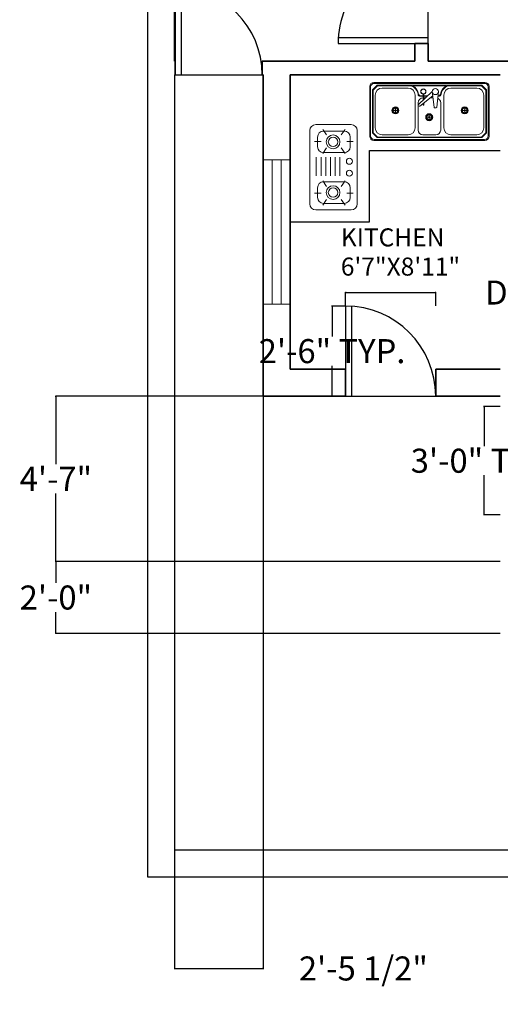
# Model space of a CAD drawing. Units: inches. Extents: x -11 to 443, y 65 to 743.
# Tile 1 of 10: x 2 to 162, y 65 to 392. Entities that reach past the tile are written whole.
import ezdxf

# ---------------------------------------------------------------- set-up
doc = ezdxf.new("R2010")
doc.units = ezdxf.units.IN
doc.header["$MEASUREMENT"] = 0
for name, color, linetype, lineweight in [('A-ANNO-DIMS', 2, 'Continuous', 18), ('A-AREA-IDEN', 2, 'Continuous', 18), ('A-DOOR', 4, 'Continuous', 25), ('A-EQPM', 8, 'Continuous', 18), ('A-FLOR-CASE', 8, 'Continuous', 25), ('A-FLOR-FIXT', 8, 'Continuous', 18), ('A-GLAZ', 4, 'Continuous', 18), ('A-WALL', 7, 'Continuous', 35), ('A-WALL-SITE', 7, 'Continuous', 30), ('C-PROP', 3, 'Continuous', 30)]:
    doc.layers.add(name, color=color, linetype=linetype, lineweight=lineweight)
doc.styles.get("Standard").update_dxf_attribs({"font": 'italic8.shx'})
doc.dimstyles.get("Standard").update_dxf_attribs({"dimtxt": 8, "dimasz": 0.18, "dimexe": 0.18, "dimexo": 0.0625, "dimgap": 0.09, "dimtad": 0, "dimtih": 1, "dimtoh": 1, "dimzin": 0, "dimdsep": 46, "dimlunit": 3, "dimtxsty": 'Standard', "dimblk": 'CLOSEDBLANK', "dimcen": 0.09, "dimclrd": 6, "dimclre": 5, "dimclrt": 4, "dimadec": 0, "dimazin": 0, "dimtfac": 1, "dimtofl": 0, "dimtmove": 0, "dimatfit": 3, "dimfxl": 1, "dimtolj": 1, "dimtzin": 0, "dimarcsym": 0})

# ---------------------------------------------------------------- blocks, each defined once
blk = doc.blocks.new('DOOR-SWING-30')
for p, q in [((0, 30), (0, 0)), ((2, 29.93), (2, 0)), ((0, 0), (30, 0))]:
    blk.add_line(p, q)
blk.add_arc((0, 0), 30, 0, 90)
blk = doc.blocks.new('WIN-48x9')
for p, q in [((0, 48), (0, 0)), ((9, 48), (0, 48)), ((3, 0), (3, 48)), ((6, 0), (6, 48)), ((9, 0), (9, 48)), ((0, 0), (9, 0))]:
    blk.add_line(p, q)
blk = doc.blocks.new('_ClosedBlank')
at = {"color": 0, "linetype": 'ByBlock', "lineweight": -2}
for p, q in [((-1, 0.17), (0, 0)), ((-1, 0.17), (-1, -0.17)), ((0, 0), (-1, -0.17))]:
    blk.add_line(p, q, dxfattribs=at)
blk = doc.blocks.new('*D20')
at = {"layer": 'A-ANNO-DIMS', "color": 5, "lineweight": -2, "transparency": 16777216}
for p, q in [((110.2, 296.98), (110.2, 301.6)), ((140.2, 296.98), (140.2, 301.6))]:
    blk.add_line(p, q, dxfattribs=at)
at = {"layer": 'A-ANNO-DIMS', "color": 6, "lineweight": -2, "transparency": 16777216}
for p, q in [((110.38, 301.42), (140.02, 301.42)), ((140.2, 301.42), (140.38, 301.42))]:
    blk.add_line(p, q, dxfattribs=at)
at = {"layer": 'Defpoints', "color": 0, "lineweight": 100, "transparency": 16777216}
for p in [(140.2, 301.42), (110.2, 296.92), (140.2, 296.92)]:
    blk.add_point(p, dxfattribs=at)
at = {"layer": 'A-ANNO-DIMS', "color": 6, "lineweight": -2, "transparency": 16777216, "xscale": 0.18, "yscale": 0.18, "zscale": 0.18, "rotation": 180}
blk.add_blockref('_ClosedBlank', (110.2, 301.42), dxfattribs=at)
at = {"layer": 'A-ANNO-DIMS', "color": 6, "lineweight": -2, "transparency": 16777216, "xscale": 0.18, "yscale": 0.18, "zscale": 0.18}
blk.add_blockref('_ClosedBlank', (140.2, 301.42), dxfattribs=at)
at = {"layer": 'A-ANNO-DIMS', "color": 4, "transparency": 16777216, "insert": (197.61, 301.42), "char_height": 8, "attachment_point": 5}
blk.add_mtext('\\A1;DOOR 2\'-6" TYP.', dxfattribs=at)
blk = doc.blocks.new('*D21')
at = {"layer": 'A-ANNO-DIMS', "color": 5, "lineweight": -2, "transparency": 16777216}
for p, q in [((110.14, 296.92), (105.52, 296.92)), ((110.14, 266.92), (105.52, 266.92))]:
    blk.add_line(p, q, dxfattribs=at)
at = {"layer": 'A-ANNO-DIMS', "color": 6, "lineweight": -2, "transparency": 16777216}
for p, q in [((105.7, 296.74), (105.7, 286.77)), ((105.7, 267.1), (105.7, 277.07))]:
    blk.add_line(p, q, dxfattribs=at)
at = {"layer": 'Defpoints', "color": 0, "lineweight": 100, "transparency": 16777216}
for p in [(105.7, 296.92), (110.2, 296.92), (110.2, 266.92)]:
    blk.add_point(p, dxfattribs=at)
at = {"layer": 'A-ANNO-DIMS', "color": 6, "lineweight": -2, "transparency": 16777216, "xscale": 0.18, "yscale": 0.18, "zscale": 0.18}
for p, rotation in [((105.7, 296.92), 90), ((105.7, 266.92), 270)]:
    blk.add_blockref('_ClosedBlank', p, dxfattribs=dict(at, rotation=rotation))
at = {"layer": 'A-ANNO-DIMS', "color": 4, "transparency": 16777216, "insert": (105.7, 281.92), "char_height": 8, "attachment_point": 5}
blk.add_mtext('\\A1;2\'-6" TYP.', dxfattribs=at)
blk = doc.blocks.new('*D23')
at = {"layer": 'A-ANNO-DIMS', "color": 5, "lineweight": -2, "transparency": 16777216}
for p, q in [((161.65, 263.44), (156.13, 263.44)), ((161.65, 227.44), (156.13, 227.44))]:
    blk.add_line(p, q, dxfattribs=at)
at = {"layer": 'A-ANNO-DIMS', "color": 6, "lineweight": -2, "transparency": 16777216}
for p, q in [((156.31, 263.26), (156.31, 250.29)), ((156.31, 227.62), (156.31, 240.59))]:
    blk.add_line(p, q, dxfattribs=at)
at = {"layer": 'Defpoints', "color": 0, "lineweight": 100, "transparency": 16777216}
for p in [(156.31, 263.44), (161.71, 263.44), (161.71, 227.44)]:
    blk.add_point(p, dxfattribs=at)
at = {"layer": 'A-ANNO-DIMS', "color": 6, "lineweight": -2, "transparency": 16777216, "xscale": 0.18, "yscale": 0.18, "zscale": 0.18}
for p, rotation in [((156.31, 263.44), 90), ((156.31, 227.44), 270)]:
    blk.add_blockref('_ClosedBlank', p, dxfattribs=dict(at, rotation=rotation))
at = {"layer": 'A-ANNO-DIMS', "color": 4, "transparency": 16777216, "insert": (156.31, 245.44), "char_height": 8, "attachment_point": 5}
blk.add_mtext('\\A1;3\'-0" TYP.', dxfattribs=at)
blk = doc.blocks.new('*D37')
at = {"layer": 'A-ANNO-DIMS', "color": 5, "lineweight": -2, "transparency": 16777216}
for p, q in [((53.21, 373.86), (53.21, 76.28)), ((82.71, 266.86), (82.71, 76.28))]:
    blk.add_line(p, q, dxfattribs=at)
at = {"layer": 'A-ANNO-DIMS', "color": 6, "lineweight": -2, "transparency": 16777216}
for p, q in [((53.39, 76.46), (82.53, 76.46)), ((82.71, 76.46), (82.89, 76.46))]:
    blk.add_line(p, q, dxfattribs=at)
at = {"layer": 'Defpoints', "color": 0, "lineweight": 100, "transparency": 16777216}
for p in [(53.21, 373.92), (82.71, 266.92), (82.71, 76.46)]:
    blk.add_point(p, dxfattribs=at)
at = {"layer": 'A-ANNO-DIMS', "color": 6, "lineweight": -2, "transparency": 16777216, "xscale": 0.18, "yscale": 0.18, "zscale": 0.18, "rotation": 180}
blk.add_blockref('_ClosedBlank', (53.21, 76.46), dxfattribs=at)
at = {"layer": 'A-ANNO-DIMS', "color": 6, "lineweight": -2, "transparency": 16777216, "xscale": 0.18, "yscale": 0.18, "zscale": 0.18}
blk.add_blockref('_ClosedBlank', (82.71, 76.46), dxfattribs=at)
at = {"layer": 'A-ANNO-DIMS', "color": 4, "transparency": 16777216, "insert": (116.12, 76.46), "char_height": 8, "attachment_point": 5}
blk.add_mtext('\\A1;2\'-5 1/2"', dxfattribs=at)
blk = doc.blocks.new('*D38')
at = {"layer": 'A-ANNO-DIMS', "color": 5, "lineweight": -2, "transparency": 16777216}
for p, q in [((82.65, 266.92), (13.57, 266.92)), ((161.65, 211.92), (13.57, 211.92))]:
    blk.add_line(p, q, dxfattribs=at)
at = {"layer": 'A-ANNO-DIMS', "color": 6, "lineweight": -2, "transparency": 16777216}
for p, q in [((13.75, 266.74), (13.75, 244.27)), ((13.75, 212.1), (13.75, 234.57))]:
    blk.add_line(p, q, dxfattribs=at)
at = {"layer": 'Defpoints', "color": 0, "lineweight": 100, "transparency": 16777216}
for p in [(82.71, 266.92), (13.75, 211.92), (161.71, 211.92)]:
    blk.add_point(p, dxfattribs=at)
at = {"layer": 'A-ANNO-DIMS', "color": 6, "lineweight": -2, "transparency": 16777216, "xscale": 0.18, "yscale": 0.18, "zscale": 0.18}
for p, rotation in [((13.75, 266.92), 90), ((13.75, 211.92), 270)]:
    blk.add_blockref('_ClosedBlank', p, dxfattribs=dict(at, rotation=rotation))
at = {"layer": 'A-ANNO-DIMS', "color": 4, "transparency": 16777216, "insert": (13.75, 239.42), "char_height": 8, "attachment_point": 5}
blk.add_mtext('\\A1;4\'-7"', dxfattribs=at)
blk = doc.blocks.new('*D39')
at = {"layer": 'A-ANNO-DIMS', "color": 5, "lineweight": -2, "transparency": 16777216}
for p, q in [((161.65, 211.92), (13.57, 211.92)), ((161.65, 187.92), (13.57, 187.92))]:
    blk.add_line(p, q, dxfattribs=at)
at = {"layer": 'A-ANNO-DIMS', "color": 6, "lineweight": -2, "transparency": 16777216}
for p, q in [((13.75, 211.74), (13.75, 204.77)), ((13.75, 188.1), (13.75, 195.07))]:
    blk.add_line(p, q, dxfattribs=at)
at = {"layer": 'Defpoints', "color": 0, "lineweight": 100, "transparency": 16777216}
for p in [(161.71, 211.92), (13.75, 187.92), (161.71, 187.92)]:
    blk.add_point(p, dxfattribs=at)
at = {"layer": 'A-ANNO-DIMS', "color": 6, "lineweight": -2, "transparency": 16777216, "xscale": 0.18, "yscale": 0.18, "zscale": 0.18}
for p, rotation in [((13.75, 211.92), 90), ((13.75, 187.92), 270)]:
    blk.add_blockref('_ClosedBlank', p, dxfattribs=dict(at, rotation=rotation))
at = {"layer": 'A-ANNO-DIMS', "color": 4, "transparency": 16777216, "insert": (13.75, 199.92), "char_height": 8, "attachment_point": 5}
blk.add_mtext('\\A1;2\'-0"', dxfattribs=at)

msp = doc.modelspace()

# ---------------------------------------------------------------- linework, layer by layer
at = {"layer": 'A-DOOR'}
for p, q in [((53.43, 402.92), (53.43, 373.92)), ((55.43, 402.851), (55.43, 373.92)), ((53.43, 373.92), (82.43, 373.92))]:
    msp.add_line(p, q, dxfattribs=at)
msp.add_arc((53.43, 373.92), 29, 0, 90, dxfattribs=at)
at = {"layer": 'A-EQPM'}
for p, q in [((100.263, 357.301), (112.074, 357.301)), ((98.294, 330.923), (98.294, 355.333)), ((102.588, 355.724), (103.876, 353.86)), ((102.838, 355.15), (109.783, 355.15)), ((110.033, 355.724), (108.744, 353.86)), ((114.042, 355.333), (114.042, 330.923)), ((99.867, 351.709), (102.015, 351.709)), ((100.869, 349.949), (100.869, 353.182)), ((112.754, 351.709), (110.606, 351.709)), ((111.751, 353.182), (111.751, 349.949)), ((102.588, 347.694), (103.876, 349.558)), ((109.783, 347.981), (102.838, 347.981)), ((110.033, 347.694), (108.744, 349.558)), ((100.44, 340.283), (100.44, 346.449)), ((102.015, 340.283), (102.015, 346.449)), ((103.589, 340.283), (103.589, 346.449)), ((105.164, 340.283), (105.164, 346.449)), ((106.739, 340.283), (106.739, 346.449)), ((108.314, 340.283), (108.314, 346.449)), ((102.588, 338.562), (103.876, 336.698)), ((109.783, 338.275), (102.838, 338.275)), ((110.033, 338.562), (108.744, 336.698)), ((99.867, 334.547), (102.015, 334.547)), ((100.869, 336.307), (100.869, 333.074)), ((112.754, 334.547), (110.606, 334.547)), ((111.751, 333.074), (111.751, 336.307)), ((102.588, 330.532), (103.876, 332.396)), ((102.838, 331.106), (109.783, 331.106)), ((110.033, 330.532), (108.744, 332.396)), ((112.074, 328.955), (100.263, 328.955))]:
    msp.add_line(p, q, dxfattribs=at)
for centre, radius in [((106.024, 351.566), 2.294), ((106.024, 351.566), 1.577), ((111.465, 345.113), 1.004), ((111.465, 341.143), 1.004), ((106.024, 334.691), 2.294), ((106.024, 334.691), 1.577)]:
    msp.add_circle(centre, radius, dxfattribs=at)
for centre, start, end in [((100.263, 355.333), 90, 180), ((112.074, 355.333), 0, 90), ((102.838, 353.182), 90, 180), ((109.783, 353.182), 0, 90), ((102.838, 349.949), 180, 270), ((109.783, 349.949), 270, 0), ((102.838, 336.307), 90, 180), ((109.783, 336.307), 0, 90), ((102.838, 333.074), 180, 270), ((109.783, 333.074), 270, 0), ((100.263, 330.923), 180, 270), ((112.074, 330.923), 270, 0)]:
    msp.add_arc(centre, 1.968, start, end, dxfattribs=at)
at = {"layer": 'A-FLOR-CASE'}
for p, q in [((118.155, 324.92), (118.155, 348.71)), ((118.155, 348.71), (161.709, 348.71)), ((91.709, 324.92), (91.709, 324.92)), ((91.709, 324.92), (118.155, 324.92))]:
    msp.add_line(p, q, dxfattribs=at)
at = {"layer": 'A-FLOR-FIXT'}
for p, q in [((120.702, 370.454), (119.127, 368.879)), ((156.607, 371.36), (119.599, 371.36)), ((156.489, 371.045), (119.718, 371.045)), ((155.505, 370.454), (120.702, 370.454)), ((157.08, 368.879), (155.505, 370.454)), ((118.221, 369.982), (118.221, 353.446)), ((118.536, 369.864), (118.536, 353.564)), ((119.127, 368.879), (119.127, 354.549)), ((120.783, 370.257), (119.324, 368.798)), ((119.324, 368.798), (119.324, 354.63)), ((120.054, 367.106), (120.054, 356.263)), ((132.049, 370.257), (120.783, 370.257)), ((130.992, 369.469), (122.416, 369.469)), ((143.821, 370.257), (132.51, 370.257)), ((133.354, 356.263), (133.354, 367.106)), ((139.065, 368.32), (134.493, 363.973)), ((135.98, 365.387), (135.98, 367.447)), ((136.226, 367.452), (136.226, 365.621)), ((139.065, 368.32), (139.64, 363.091)), ((140.598, 363.093), (141.117, 368.32)), ((142.9, 367.106), (142.9, 356.263)), ((155.423, 370.257), (144.283, 370.257)), ((153.838, 369.469), (145.263, 369.469)), ((156.883, 368.798), (155.423, 370.257)), ((156.201, 356.263), (156.201, 367.106)), ((156.883, 354.63), (156.883, 368.798)), ((157.08, 354.549), (157.08, 368.879)), ((157.67, 353.564), (157.67, 369.864)), ((157.985, 353.446), (157.985, 369.982)), ((134.356, 364.61), (134.356, 355.478)), ((139.227, 366.841), (134.924, 363.473)), ((135.98, 366.938), (135.095, 366.938)), ((135.98, 366.741), (135.095, 366.741)), ((135.98, 366.185), (135.931, 366.185)), ((135.98, 363.759), (135.98, 364.299)), ((136.226, 363.759), (135.98, 363.759)), ((137.612, 366.938), (136.226, 366.938)), ((137.405, 366.741), (136.226, 366.741)), ((136.819, 366.185), (136.226, 366.185)), ((136.226, 364.492), (136.226, 363.759)), ((139.3, 366.185), (138.389, 366.185)), ((139.238, 366.741), (139.1, 366.741)), ((141.237, 366.741), (140.96, 366.741)), ((141.237, 366.938), (140.98, 366.938)), ((141.862, 355.478), (141.862, 364.61)), ((126.58, 362.025), (125.989, 362.025)), ((126.784, 362.229), (126.784, 362.819)), ((126.784, 361.821), (126.784, 361.23)), ((126.988, 362.025), (127.578, 362.025)), ((134.486, 363.521), (134.466, 363.545)), ((138.031, 359.981), (138.031, 360.571)), ((139.836, 362.916), (140.402, 362.915)), ((149.638, 362.025), (149.047, 362.025)), ((149.842, 362.229), (149.842, 362.819)), ((149.842, 361.821), (149.842, 361.23)), ((150.045, 362.025), (150.636, 362.025)), ((137.828, 359.777), (137.237, 359.777)), ((138.031, 359.573), (138.031, 358.982)), ((138.235, 359.777), (138.826, 359.777)), ((119.127, 354.549), (120.702, 352.974)), ((119.324, 354.63), (120.783, 353.171)), ((155.423, 353.171), (156.883, 354.63)), ((155.505, 352.974), (157.08, 354.549)), ((119.599, 352.068), (156.607, 352.068)), ((119.718, 352.383), (156.489, 352.383)), ((120.702, 352.974), (155.505, 352.974)), ((120.783, 353.171), (155.423, 353.171)), ((122.416, 353.9), (130.992, 353.9)), ((135.931, 353.903), (140.288, 353.903)), ((145.263, 353.9), (153.838, 353.9))]:
    msp.add_line(p, q, dxfattribs=at)
for centre, radius in [((136.083, 368.307), 0.866), ((136.083, 368.307), 0.787), ((140.091, 368.32), 1.026), ((126.784, 362.025), 1.162), ((126.784, 362.025), 1.099), ((126.784, 362.025), 0.83), ((126.784, 362.025), 0.794), ((126.784, 362.025), 0.204), ((126.784, 362.025), 0.0958), ((138.031, 359.777), 1.162), ((138.031, 359.777), 1.099), ((138.031, 359.777), 0.83), ((138.031, 359.777), 0.794), ((149.842, 362.025), 1.162), ((149.842, 362.025), 1.099), ((149.842, 362.025), 0.83), ((149.842, 362.025), 0.794), ((149.842, 362.025), 0.204), ((149.842, 362.025), 0.0958), ((138.031, 359.777), 0.204), ((138.031, 359.777), 0.0958)]:
    msp.add_circle(centre, radius, dxfattribs=at)
for centre, radius, start, end in [((119.599, 369.982), 1.378, 90, 180), ((119.718, 369.864), 1.181, 90, 180), ((156.489, 369.864), 1.181, 0, 90), ((156.607, 369.982), 1.378, 0, 90), ((122.416, 367.106), 2.362, 90, 180), ((130.992, 367.106), 2.362, 0, 90), ((130.657, 366.822), 3.706, 9.04683, 67.9454), ((130.657, 366.822), 3.903, 9.04683, 61.65237), ((135.095, 367.529), 0.787, 189.04683, 270), ((135.095, 367.529), 0.591, 189.04683, 270), ((141.237, 367.529), 0.591, 270, 350.95317), ((141.237, 367.529), 0.787, 270, 350.95317), ((145.674, 366.822), 3.903, 118.34763, 170.95317), ((145.674, 366.822), 3.706, 112.0546, 170.95317), ((145.263, 367.106), 2.362, 90, 180), ((153.838, 367.106), 2.362, 0, 90), ((135.931, 364.61), 1.575, 90, 180), ((134.71, 363.745), 0.315, 133.56108, 219.26187), ((140.288, 364.61), 1.575, 360, 67.38374), ((134.73, 363.721), 0.315, 219.26187, 308.04948), ((139.836, 363.113), 0.197, 186.28076, 269.95427), ((140.402, 363.112), 0.197, 269.95427, 354.32947), ((122.416, 356.263), 2.362, 180, 270), ((130.992, 356.263), 2.362, 270, 0), ((135.931, 355.478), 1.575, 180, 270), ((140.288, 355.478), 1.575, 270, 0), ((145.263, 356.263), 2.362, 180, 270), ((153.838, 356.263), 2.362, 270, 0), ((119.599, 353.446), 1.378, 180, 270), ((119.718, 353.564), 1.181, 180, 270), ((156.489, 353.564), 1.181, 270, 360), ((156.607, 353.446), 1.378, 270, 360)]:
    msp.add_arc(centre, radius, start, end, dxfattribs=at)
at = {"layer": 'A-WALL'}
for p, q in [((53.209, 517.92), (53.209, 378.42)), ((137.709, 384.35), (133.209, 384.35)), ((133.209, 384.35), (133.209, 378.42)), ((137.709, 384.35), (137.709, 378.42)), ((53.209, 378.42), (53.43, 378.42)), ((53.43, 373.92), (53.43, 378.42)), ((82.43, 373.92), (82.43, 378.42)), ((82.43, 378.42), (133.209, 378.42)), ((137.709, 378.42), (169.908, 378.42)), ((53.209, 373.92), (53.43, 373.92)), ((82.709, 373.92), (82.43, 373.92)), ((82.43, 373.92), (82.709, 373.92)), ((82.709, 266.92), (82.709, 373.92)), ((91.709, 275.92), (91.709, 373.92)), ((91.709, 373.92), (161.709, 373.92)), ((91.709, 275.92), (110.201, 275.92)), ((110.201, 275.92), (110.201, 266.92)), ((140.201, 275.92), (140.201, 266.92)), ((140.201, 275.92), (161.709, 275.92)), ((82.709, 266.92), (110.201, 266.92)), ((140.201, 266.92), (161.709, 266.92))]:
    msp.add_line(p, q, dxfattribs=at)
at = {"layer": 'A-WALL-SITE'}
for p, q in [((53.209, 373.92), (53.209, 115.92)), ((53.209, 115.92), (323.209, 115.92))]:
    msp.add_line(p, q, dxfattribs=at)
at = {"layer": 'C-PROP'}
msp.add_lwpolyline([(44.209, 106.92), (332.209, 106.92), (332.209, 706.92), (44.209, 706.92)], close=True, dxfattribs=at)

# ---------------------------------------------------------------- block references
at = {"layer": 'A-DOOR', "rotation": 89.99999999999991}
msp.add_blockref('DOOR-SWING-30', (137.709, 384.35), dxfattribs=at)
at = {"layer": 'A-DOOR'}
msp.add_blockref('DOOR-SWING-30', (110.201, 266.92), dxfattribs=at)
at = {"layer": 'A-GLAZ'}
msp.add_blockref('WIN-48x9', (82.709, 297.576), dxfattribs=at)

# ---------------------------------------------------------------- texts
at = {"layer": 'A-AREA-IDEN'}
for s, p in [('KITCHEN', (108.605, 316.776)), ('6\'7"X8\'11"', (108.605, 307.062))]:
    msp.add_text(s, height=6, dxfattribs=at).set_placement(p)

# ---------------------------------------------------------------- dimensions: what is measured, and where the dimension line sits
at = {"layer": 'A-ANNO-DIMS'}
dim = msp.add_linear_dim(base=(82.709, 76.46), p1=(53.209, 373.92), p2=(82.709, 266.92), dimstyle='Standard', override={"dimdec": 1, "dimlfac": 1, "dimrnd": 0, "dimzin": 1, "dimdsep": 46, "dimlunit": 4, "dimfrac": 2}, dxfattribs=at)
dim.commit()
dim.dimension.update_dxf_attribs({"geometry": '*D37', "text_midpoint": (116.122, 76.46)})
dim = msp.add_linear_dim(base=(140.201, 301.42), p1=(110.201, 296.92), p2=(140.201, 296.92), text='DOOR <> TYP.', dimstyle='Standard', override={"dimdec": 1, "dimlfac": 1, "dimrnd": 0, "dimzin": 1, "dimdsep": 46, "dimlunit": 4, "dimfrac": 2}, dxfattribs=at)
dim.commit()
dim.dimension.update_dxf_attribs({"geometry": '*D20', "text_midpoint": (197.614, 301.42)})
for base, p1, p2, picture, middle in [((105.701, 296.92), (110.201, 266.92), (110.201, 296.92), '*D21', (105.701, 281.92)), ((156.309, 263.442), (161.709, 227.442), (161.709, 263.442), '*D23', (156.309, 245.442))]:
    dim = msp.add_linear_dim(base=base, p1=p1, p2=p2, angle=90, text='<> TYP.', dimstyle='Standard', override={"dimdec": 1, "dimlfac": 1, "dimrnd": 0, "dimzin": 1, "dimdsep": 46, "dimlunit": 4, "dimfrac": 2}, dxfattribs=at)
    dim.commit()
    dim.dimension.update_dxf_attribs({"geometry": picture, "text_midpoint": middle})
for base, p1, p2, picture, middle in [((13.75, 211.92), (82.709, 266.92), (161.709, 211.92), '*D38', (13.75, 239.42)), ((13.75, 187.92), (161.709, 211.92), (161.709, 187.92), '*D39', (13.75, 199.92))]:
    dim = msp.add_linear_dim(base=base, p1=p1, p2=p2, angle=90, dimstyle='Standard', override={"dimdec": 1, "dimlfac": 1, "dimrnd": 0, "dimzin": 1, "dimdsep": 46, "dimlunit": 4, "dimfrac": 2}, dxfattribs=at)
    dim.commit()
    dim.dimension.update_dxf_attribs({"geometry": picture, "text_midpoint": middle})

doc.saveas('drawing.dxf')
